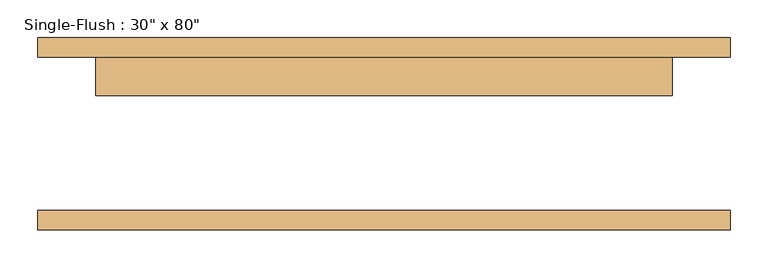
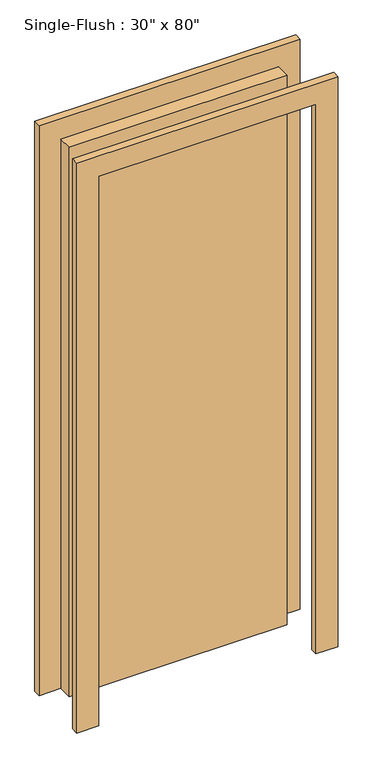
"""IFC4 building model written with IfcOpenShell, lengths in millimetres: door geometry."""

from ifc_helpers import new_model, si_unit, frame, origin, origin_with_axes, place, context, project, spatial, polyline, outline, extrude, source, transform, mapped, element, save


def door_fadea3f2(model_context):
    return source(origin(), model_context, "Body", "SweptSolid", [
        extrude(outline(polyline([(2108.2, -457.2), (0.0, -457.2), (0.0, -381.0), (2032.0, -381.0), (2032.0, 381.0), (0.0, 381.0), (0.0, 457.2), (2108.2, 457.2), (2108.2, -457.2)])), frame((0.0, 101.6, 0.0), z_axis=(0.0, 1.0, 0.0), x_axis=(0.0, 0.0, 1.0)), (0.0, 0.0, 1.0), 25.4),
        extrude(outline(polyline([(2108.2, 457.2), (2108.2, -457.2), (0.0, -457.2), (0.0, -381.0), (2032.0, -381.0), (2032.0, 381.0), (0.0, 381.0), (0.0, 457.2), (2108.2, 457.2)])), frame((0.0, -127.0, 0.0), z_axis=(0.0, 1.0, 0.0), x_axis=(0.0, 0.0, 1.0)), (0.0, 0.0, 1.0), 25.4),
        extrude(outline(polyline([(381.0, 50.8), (-381.0, 50.8), (-381.0, 101.6), (381.0, 101.6), (381.0, 50.8)])), origin_with_axes(), (0.0, 0.0, 1.0), 2032.0),
    ])


if __name__ == "__main__":
    model = new_model("IFC4")
    model_context = context("Model", 3, world=origin())
    ifc_project = project(units=[si_unit("LENGTHUNIT", "METRE", prefix="MILLI")], contexts=[model_context])
    site = spatial("IfcSite", under=ifc_project)
    building = spatial("IfcBuilding", under=site)
    placement = place(None, origin())
    door_shape = door_fadea3f2(model_context)
    element("IfcDoor", 1, ObjectType="Single-Flush : 30\" x 80\"", at=placement, inside=building, context=model_context, shape_type="MappedRepresentation", body=[
        mapped(door_shape, transform((0.0, 0.0, 0.0), x_axis=(1.0, 0.0, 0.0), y_axis=(0.0, 1.0, 0.0), z_axis=(0.0, 0.0, 1.0))),
    ])
    save(model, "model.ifc")

# Revit data of these elements
# Type "Single-Flush : 30\" x 80\""
#   Type Mark = "5"
#   Construction Type Id = "MDOOR"
#   Assembly Code = "C1020"
#   Analytic Construction = "Metal"
#   Thickness = 0' - 2"
#   Heat Transfer Coefficient (U) = 0.651978 BTU/(h·ft²·°F)
#   Height = 6' - 8"
#   Trim Projection Ext = 0' - 1"
#   Trim Projection Int = 0' - 1"
#   Trim Width = 0' - 3"
#   Width = 2' - 6"
#   Define Thermal Properties by = 1
#   Define Thermal Properties by = 1
#   Door Material = Door - Panel
#   Frame Material = Door - Frame
#   Visual Light Transmittance = 0
#   Solar Heat Gain Coefficient = 0
#   Function = (empty or 0)
#   Wall Closure = (empty or 0)
# Element 1 (IfcDoor, "Single-Flush : 30\" x 80\"")
#   Materials on its faces: "Door - Frame", "Door - Panel"
# Materials
#   "Door - Panel": class "Wood", colour RGB 210 159 95, transparency 0, Cost = 0
#   "Door - Frame": colour RGB 118 70 51, transparency 0, Cost = 0
